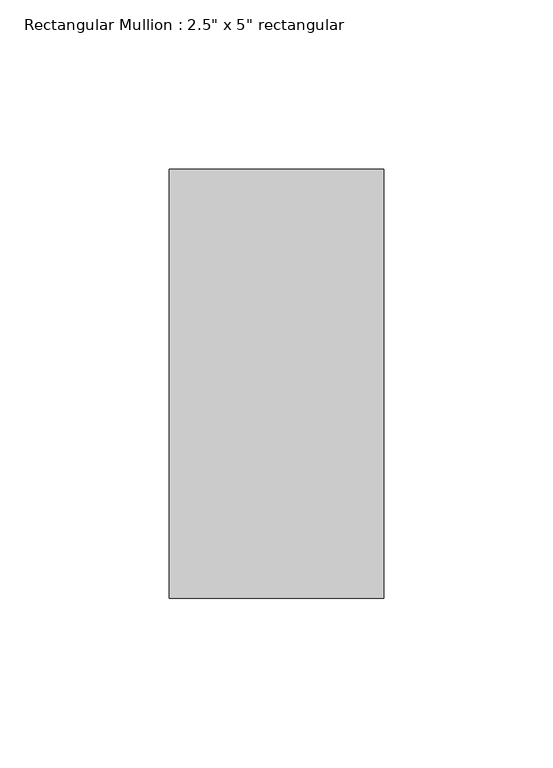
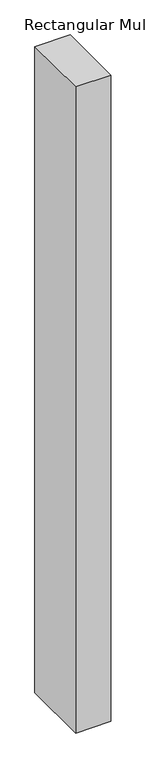
"""IFC4 building model written with IfcOpenShell, lengths in millimetres: member geometry."""

from ifc_helpers import new_model, si_unit, frame, origin, place, context, project, spatial, polyline, outline, extrude, source, transform, mapped, element, save


def member_a972b4dd(model_context):
    return source(origin(), model_context, "Body", "SweptSolid", [
        extrude(outline(polyline([(31.75, 63.5), (31.75, -63.5), (-31.75, -63.5), (-31.75, 63.5), (31.75, 63.5)])), frame((0.0, 0.0, -1231.8999998), z_axis=(0.0, 0.0, 1.0), x_axis=(1.0, 0.0, 0.0)), (0.0, 0.0, 1.0), 1231.8999998),
    ])


if __name__ == "__main__":
    model = new_model("IFC4")
    model_context = context("Model", 3, world=origin())
    ifc_project = project(units=[si_unit("LENGTHUNIT", "METRE", prefix="MILLI")], contexts=[model_context])
    site = spatial("IfcSite", under=ifc_project)
    building = spatial("IfcBuilding", under=site)
    placement = place(None, origin())
    member_shape = member_a972b4dd(model_context)
    element("IfcMember", 1, ObjectType="Rectangular Mullion : 2.5\" x 5\" rectangular", at=placement, inside=building, context=model_context, shape_type="MappedRepresentation", body=[
        mapped(member_shape, transform((0.0, 0.0, 0.0), x_axis=(1.0, 0.0, 0.0), y_axis=(0.0, 1.0, 0.0), z_axis=(0.0, 0.0, 1.0))),
    ])
    save(model, "model.ifc")

# Revit data of these elements
# Type "Rectangular Mullion : 2.5\" x 5\" rectangular"
#   built-in parameter 1007304 = 0.416667 (stored number, unit not read)
#   built-in parameter 1007301 = 0.104167 (stored number, unit not read)
#   built-in parameter 1007300 = 0.104167 (stored number, unit not read)
# Element 1 (IfcMember, "Rectangular Mullion : 2.5\" x 5\" rectangular")
#   Materials on its faces: "Aluminum"
# Materials
#   "Aluminum": class "Metal", colour RGB 247 247 247, transparency 0, Description = "Aluminum 6061", Cost = 0
